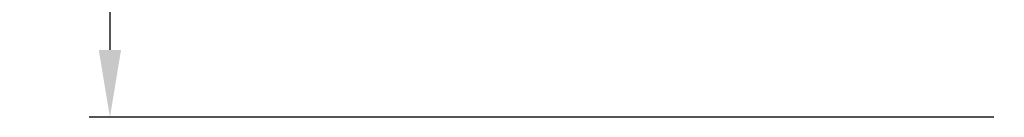
# Model space of a CAD drawing. Units: inches. Extents: x 2091 to 2899, y 967 to 2217.
# Tile 1 of 256: x 2120 to 2179, y 1091 to 1096. Entities that reach past the tile are written whole.
import ezdxf

# ---------------------------------------------------------------- set-up
doc = ezdxf.new("R2010")
doc.units = ezdxf.units.IN
doc.layers.add('A-ANNO-DIMS', color=2, linetype='Continuous', lineweight=18)
doc.styles.get("Standard").update_dxf_attribs({"font": 'arial.ttf'})
doc.dimstyles.new('ISO-25', dxfattribs={"dimtxt": 4, "dimasz": 4, "dimexe": 1.25, "dimexo": 0.625, "dimtad": 1, "dimdec": 0, "dimlunit": 3, "dimtxsty": 'Standard', "dimcen": 2.5, "dimadec": 0, "dimazin": 0, "dimtfac": 1, "dimtdec": 0, "dimtmove": 0, "dimatfit": 3, "dimfxl": 1, "dimarcsym": 0})

# ---------------------------------------------------------------- blocks, each defined once
blk = doc.blocks.new('*D32')
at = {"layer": 'A-ANNO-DIMS', "color": 0, "lineweight": -2, "transparency": 16777216}
for p, q in [((2178.68, 2050.678), (2124.594, 2050.678)), ((2125.844, 2046.678), (2125.844, 1094.678)), ((2178.68, 1090.678), (2124.594, 1090.678))]:
    blk.add_line(p, q, dxfattribs=at)
at = {"layer": 'A-ANNO-DIMS', "color": 0, "transparency": 16777216}
for points in [[(2125.177, 2046.678), (2126.511, 2046.678), (2125.844, 2050.678)], [(2125.177, 1094.678), (2126.511, 1094.678), (2125.844, 1090.678)]]:
    blk.add_solid(points, dxfattribs=at)
at = {"layer": 'Defpoints', "color": 0, "transparency": 16777216}
for p in [(2179.305, 2050.678), (2125.844, 1090.678), (2179.305, 1090.678)]:
    blk.add_point(p, dxfattribs=at)
at = {"layer": 'A-ANNO-DIMS', "color": 0, "transparency": 16777216, "insert": (2123.177, 1570.678), "char_height": 4, "attachment_point": 5, "rotation": 90}
blk.add_mtext("80'", dxfattribs=at)

msp = doc.modelspace()

# ---------------------------------------------------------------- dimensions: what is measured, and where the dimension line sits
at = {"layer": 'A-ANNO-DIMS'}
dim = msp.add_linear_dim(base=(2125.844, 1090.678), p1=(2179.305, 2050.678), p2=(2179.305, 1090.678), angle=90, dimstyle='ISO-25', override={"dimclrd": 0, "dimclre": 0, "dimclrt": 0}, dxfattribs=at)
dim.commit()
dim.dimension.update_dxf_attribs({"geometry": '*D32', "text_midpoint": (2123.177, 1570.678)})

doc.saveas('drawing.dxf')
